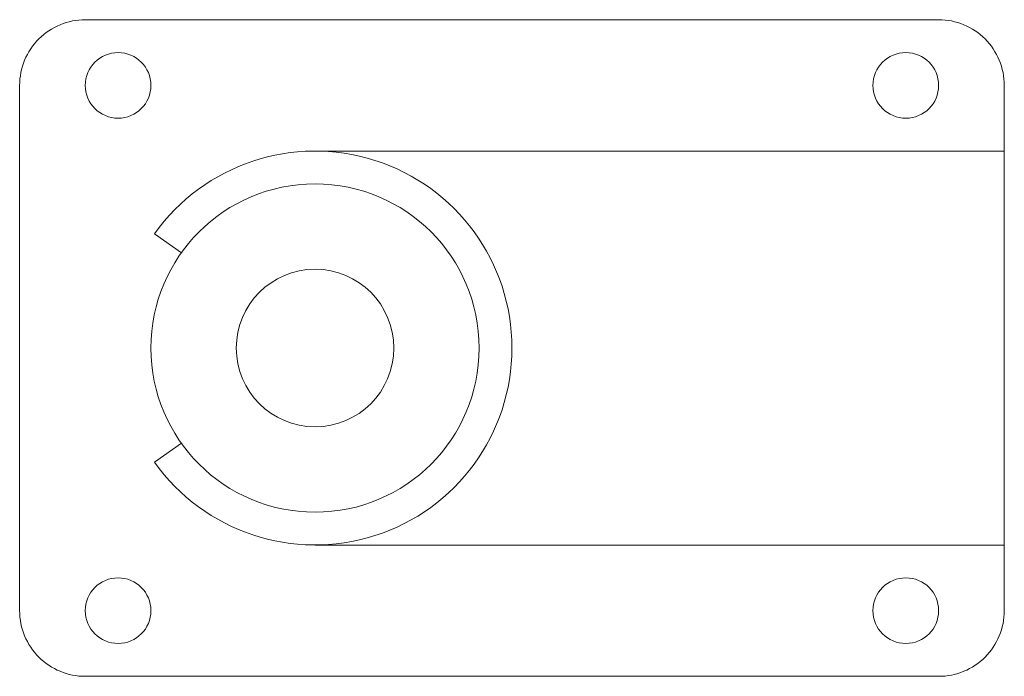
# Model space of a CAD drawing. Units: millimetres. Extents: x 3316 to 3466, y 2624 to 2724.
import ezdxf

# ---------------------------------------------------------------- set-up
doc = ezdxf.new("R2010")
doc.units = ezdxf.units.MM
doc.layers.add('M-CONS', color=8, linetype='Continuous', lineweight=18)

msp = doc.modelspace()

# ---------------------------------------------------------------- linework, layer by layer
at = {"layer": 'M-CONS'}
msp.add_lwpolyline([(3326.49, 2623.67), (3456.49, 2623.67, 0.414214), (3466.49, 2633.67), (3466.49, 2713.67, 0.414214), (3456.49, 2723.67), (3326.49, 2723.67, 0.414214), (3316.49, 2713.67), (3316.49, 2633.67, 0.414214)], format="xyb", close=True, dxfattribs=at)
msp.add_lwpolyline([(3341.12, 2659.19), (3337.04, 2656.29, 3.132804), (3337.04, 2691.05), (3341.12, 2688.16)], format="xyb", dxfattribs=at)
msp.add_lwpolyline([(3361.49, 2643.67), (3466.49, 2643.67), (3466.49, 2703.67), (3361.49, 2703.67)], dxfattribs=at)
for centre, radius in [((3331.49, 2713.67), 5), ((3451.49, 2713.67), 5), ((3361.49, 2673.67), 25), ((3361.49, 2673.67), 12), ((3331.49, 2633.67), 5), ((3451.49, 2633.67), 5)]:
    msp.add_circle(centre, radius, dxfattribs=at)

doc.saveas('drawing.dxf')
